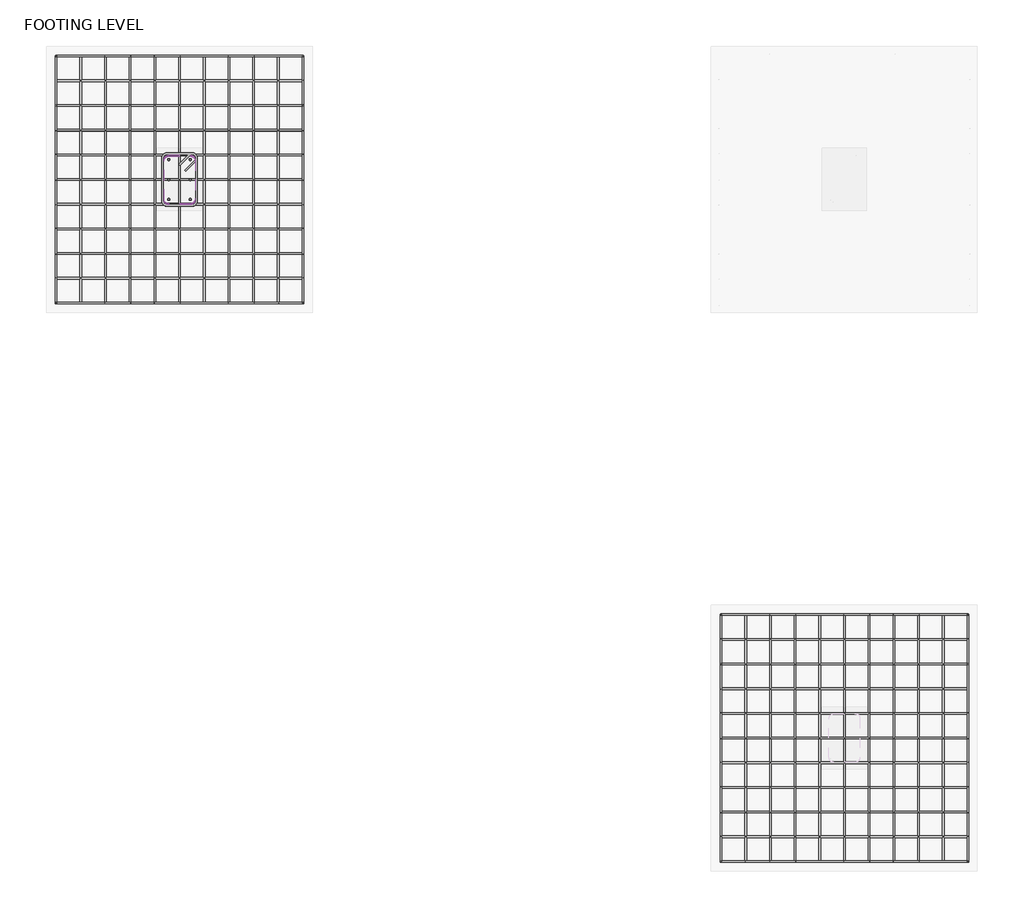
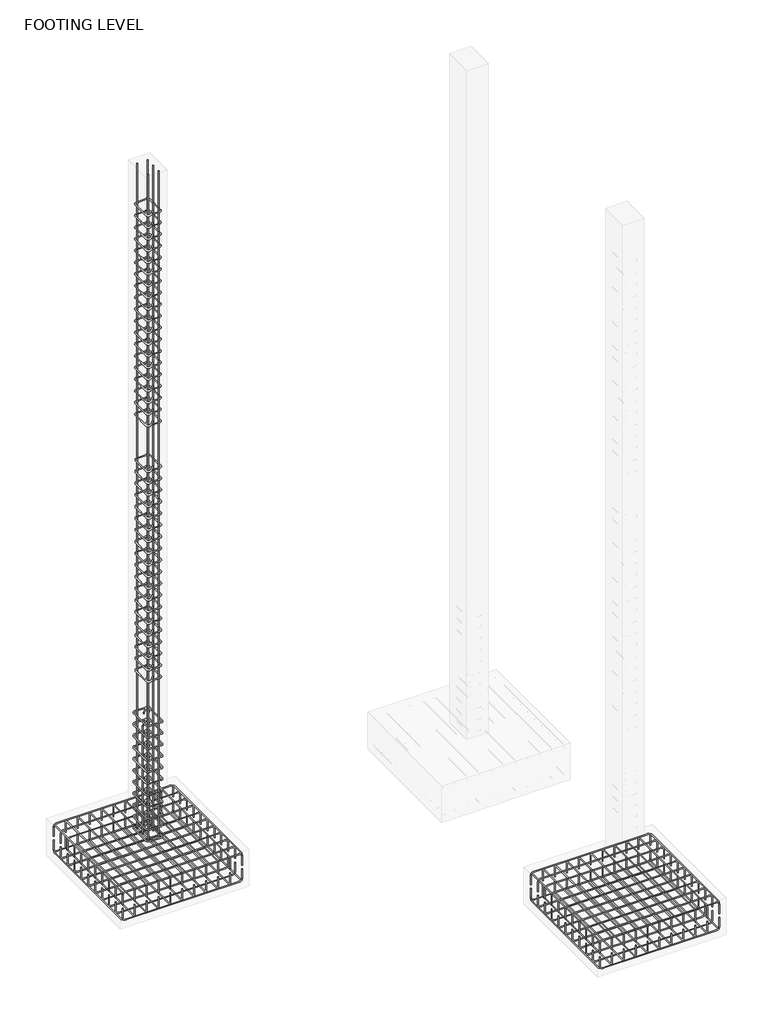
# One storey, part 2 of 9: 17 reinforcing bars.
"""IFC4 building model written with IfcOpenShell, lengths in millimetres."""

from ifc_helpers import new_model, si_unit, point, frame, origin, place, context, project, spatial, polyline, circle_curve, trimmed, segment, composite_curve, source, transform, mapped, element, save
from ifc_brep_helpers import swept_disk

model = new_model("IFC4")

# Units and contexts
model_context = context("Model", 3, world=origin())
ifc_project = project(units=[si_unit("LENGTHUNIT", "METRE", prefix="MILLI")], contexts=[model_context])

# Site, building, storey
site = spatial("IfcSite", under=ifc_project)
building = spatial("IfcBuilding", under=site)
storey = spatial("IfcBuildingStorey", under=building, Name="FOOTING LEVEL", Elevation=-1981.2)

# Reinforcing bars
placement = place(None, origin())
reinforcing_bar_shape = source(origin(), model_context, "Body", "SolidModel", [
    swept_disk(composite_curve([segment(polyline([(-7844.8521159, -3054.1904098, -2183.60625), (-7844.8521159, -3054.1904098, -2069.30625)]), True, "CONTINUOUS"), segment(trimmed(circle_curve(frame((-7844.8521159, -3087.5279098, -2069.30625), z_axis=(1.0, 0.0, 0.0), x_axis=(0.0, 33.33750000000009, 0.0)), 33.3375), [point((-7844.8521159, -3054.1904098, -2069.30625))], [point((-7844.8521159, -3087.5279098, -2035.96875))], True, "CARTESIAN"), True, "CONTINUOUS"), segment(polyline([(-7844.8521159, -3087.5279098, -2035.96875), (-7844.8521159, -4435.3154098, -2035.96875)]), True, "CONTINUOUS"), segment(trimmed(circle_curve(frame((-7844.8521159, -4435.3154098, -2069.30625), z_axis=(1.0, 0.0, 0.0), x_axis=(0.0, 0.0, 33.33750000000009)), 33.3375), [point((-7844.8521159, -4435.3154098, -2035.96875))], [point((-7844.8521159, -4468.6529098, -2069.30625))], True, "CARTESIAN"), True, "CONTINUOUS"), segment(polyline([(-7844.8521159, -4468.6529098, -2069.30625), (-7844.8521159, -4468.6529098, -2183.60625)]), True, "CONTINUOUS")], self_intersect=False), 4.7625),
])
element("IfcReinforcingBar", 1, at=placement, inside=storey, context=model_context, shape_type="MappedRepresentation", body=[
    mapped(reinforcing_bar_shape, transform((0.0, 0.0, 0.0), x_axis=(1.0, 0.0, 0.0), y_axis=(0.0, 1.0, 0.0), z_axis=(0.0, 0.0, 1.0))),
    mapped(reinforcing_bar_shape, transform((-141.44625, 0.0, 0.0), x_axis=(1.0, 0.0, 0.0), y_axis=(0.0, 1.0, 0.0), z_axis=(0.0, 0.0, 1.0))),
    mapped(reinforcing_bar_shape, transform((-282.8925, 0.0, 0.0), x_axis=(1.0, 0.0, 0.0), y_axis=(0.0, 1.0, 0.0), z_axis=(0.0, 0.0, 1.0))),
    mapped(reinforcing_bar_shape, transform((-424.33875, 0.0, 0.0), x_axis=(1.0, 0.0, 0.0), y_axis=(0.0, 1.0, 0.0), z_axis=(0.0, 0.0, 1.0))),
    mapped(reinforcing_bar_shape, transform((-565.785, 0.0, 0.0), x_axis=(1.0, 0.0, 0.0), y_axis=(0.0, 1.0, 0.0), z_axis=(0.0, 0.0, 1.0))),
    mapped(reinforcing_bar_shape, transform((-707.23125, 0.0, 0.0), x_axis=(1.0, 0.0, 0.0), y_axis=(0.0, 1.0, 0.0), z_axis=(0.0, 0.0, 1.0))),
    mapped(reinforcing_bar_shape, transform((-848.6775, 0.0, 0.0), x_axis=(1.0, 0.0, 0.0), y_axis=(0.0, 1.0, 0.0), z_axis=(0.0, 0.0, 1.0))),
    mapped(reinforcing_bar_shape, transform((-990.12375, 0.0, 0.0), x_axis=(1.0, 0.0, 0.0), y_axis=(0.0, 1.0, 0.0), z_axis=(0.0, 0.0, 1.0))),
    mapped(reinforcing_bar_shape, transform((-1131.57, 0.0, 0.0), x_axis=(1.0, 0.0, 0.0), y_axis=(0.0, 1.0, 0.0), z_axis=(0.0, 0.0, 1.0))),
    mapped(reinforcing_bar_shape, transform((-1273.01625, 0.0, 0.0), x_axis=(1.0, 0.0, 0.0), y_axis=(0.0, 1.0, 0.0), z_axis=(0.0, 0.0, 1.0))),
    mapped(reinforcing_bar_shape, transform((-1414.4625, 0.0, 0.0), x_axis=(1.0, 0.0, 0.0), y_axis=(0.0, 1.0, 0.0), z_axis=(0.0, 0.0, 1.0))),
])
reinforcing_bar_2_shape = source(origin(), model_context, "Body", "SolidModel", [
    swept_disk(composite_curve([segment(polyline([(-7844.8521159, -4468.6529098, -2235.99375), (-7844.8521159, -4468.6529098, -2350.29375)]), True, "CONTINUOUS"), segment(trimmed(circle_curve(frame((-7844.8521159, -4435.3154098, -2350.29375), z_axis=(1.0, 0.0, 0.0), x_axis=(0.0, -33.337499999999636, 0.0)), 33.3375), [point((-7844.8521159, -4468.6529098, -2350.29375))], [point((-7844.8521159, -4435.3154098, -2383.63125))], True, "CARTESIAN"), True, "CONTINUOUS"), segment(polyline([(-7844.8521159, -4435.3154098, -2383.63125), (-7844.8521159, -3087.5279098, -2383.63125)]), True, "CONTINUOUS"), segment(trimmed(circle_curve(frame((-7844.8521159, -3087.5279098, -2350.29375), z_axis=(1.0, 0.0, 0.0), x_axis=(0.0, 0.0, -33.33750000000009)), 33.3375), [point((-7844.8521159, -3087.5279098, -2383.63125))], [point((-7844.8521159, -3054.1904098, -2350.29375))], True, "CARTESIAN"), True, "CONTINUOUS"), segment(polyline([(-7844.8521159, -3054.1904098, -2350.29375), (-7844.8521159, -3054.1904098, -2235.99375)]), True, "CONTINUOUS")], self_intersect=False), 4.7625),
])
element("IfcReinforcingBar", 2, at=placement, inside=storey, context=model_context, shape_type="MappedRepresentation", body=[
    mapped(reinforcing_bar_2_shape, transform((0.0, 0.0, 0.0), x_axis=(1.0, 0.0, 0.0), y_axis=(0.0, 1.0, 0.0), z_axis=(0.0, 0.0, 1.0))),
    mapped(reinforcing_bar_2_shape, transform((-141.44625, 0.0, 0.0), x_axis=(1.0, 0.0, 0.0), y_axis=(0.0, 1.0, 0.0), z_axis=(0.0, 0.0, 1.0))),
    mapped(reinforcing_bar_2_shape, transform((-282.8925, 0.0, 0.0), x_axis=(1.0, 0.0, 0.0), y_axis=(0.0, 1.0, 0.0), z_axis=(0.0, 0.0, 1.0))),
    mapped(reinforcing_bar_2_shape, transform((-424.33875, 0.0, 0.0), x_axis=(1.0, 0.0, 0.0), y_axis=(0.0, 1.0, 0.0), z_axis=(0.0, 0.0, 1.0))),
    mapped(reinforcing_bar_2_shape, transform((-565.785, 0.0, 0.0), x_axis=(1.0, 0.0, 0.0), y_axis=(0.0, 1.0, 0.0), z_axis=(0.0, 0.0, 1.0))),
    mapped(reinforcing_bar_2_shape, transform((-707.23125, 0.0, 0.0), x_axis=(1.0, 0.0, 0.0), y_axis=(0.0, 1.0, 0.0), z_axis=(0.0, 0.0, 1.0))),
    mapped(reinforcing_bar_2_shape, transform((-848.6775, 0.0, 0.0), x_axis=(1.0, 0.0, 0.0), y_axis=(0.0, 1.0, 0.0), z_axis=(0.0, 0.0, 1.0))),
    mapped(reinforcing_bar_2_shape, transform((-990.12375, 0.0, 0.0), x_axis=(1.0, 0.0, 0.0), y_axis=(0.0, 1.0, 0.0), z_axis=(0.0, 0.0, 1.0))),
    mapped(reinforcing_bar_2_shape, transform((-1131.57, 0.0, 0.0), x_axis=(1.0, 0.0, 0.0), y_axis=(0.0, 1.0, 0.0), z_axis=(0.0, 0.0, 1.0))),
    mapped(reinforcing_bar_2_shape, transform((-1273.01625, 0.0, 0.0), x_axis=(1.0, 0.0, 0.0), y_axis=(0.0, 1.0, 0.0), z_axis=(0.0, 0.0, 1.0))),
    mapped(reinforcing_bar_2_shape, transform((-1414.4625, 0.0, 0.0), x_axis=(1.0, 0.0, 0.0), y_axis=(0.0, 1.0, 0.0), z_axis=(0.0, 0.0, 1.0))),
])
reinforcing_bar_3_shape = source(origin(), model_context, "Body", "SolidModel", [
    swept_disk(composite_curve([segment(polyline([(-9259.3146159, -3054.1904098, -2183.5650752), (-9259.3146159, -3054.1904098, -2069.2650752)]), True, "CONTINUOUS"), segment(trimmed(circle_curve(frame((-9225.9771159, -3054.1904098, -2069.2650752), z_axis=(0.0, 1.0, 0.0), x_axis=(-33.337500000001455, 0.0, 0.0)), 33.3375), [point((-9259.3146159, -3054.1904098, -2069.2650752))], [point((-9225.9771159, -3054.1904098, -2035.9275752))], True, "CARTESIAN"), True, "CONTINUOUS"), segment(polyline([(-9225.9771159, -3054.1904098, -2035.9275752), (-7878.1896159, -3054.1904098, -2035.9275752)]), True, "CONTINUOUS"), segment(trimmed(circle_curve(frame((-7878.1896159, -3054.1904098, -2069.2650752), z_axis=(0.0, 1.0, 0.0), x_axis=(0.0, 0.0, 33.337499999999864)), 33.3375), [point((-7878.1896159, -3054.1904098, -2035.9275752))], [point((-7844.8521159, -3054.1904098, -2069.2650752))], True, "CARTESIAN"), True, "CONTINUOUS"), segment(polyline([(-7844.8521159, -3054.1904098, -2069.2650752), (-7844.8521159, -3054.1904098, -2183.5650752)]), True, "CONTINUOUS")], self_intersect=False), 4.7625),
])
element("IfcReinforcingBar", 3, at=placement, inside=storey, context=model_context, shape_type="MappedRepresentation", body=[
    mapped(reinforcing_bar_3_shape, transform((0.0, 0.0, 0.0), x_axis=(1.0, 0.0, 0.0), y_axis=(0.0, 1.0, 0.0), z_axis=(0.0, 0.0, 1.0))),
    mapped(reinforcing_bar_3_shape, transform((0.0, -141.44625, 0.0), x_axis=(1.0, 0.0, 0.0), y_axis=(0.0, 1.0, 0.0), z_axis=(0.0, 0.0, 1.0))),
    mapped(reinforcing_bar_3_shape, transform((0.0, -282.8925, 0.0), x_axis=(1.0, 0.0, 0.0), y_axis=(0.0, 1.0, 0.0), z_axis=(0.0, 0.0, 1.0))),
    mapped(reinforcing_bar_3_shape, transform((0.0, -424.33875, 0.0), x_axis=(1.0, 0.0, 0.0), y_axis=(0.0, 1.0, 0.0), z_axis=(0.0, 0.0, 1.0))),
    mapped(reinforcing_bar_3_shape, transform((0.0, -565.785, 0.0), x_axis=(1.0, 0.0, 0.0), y_axis=(0.0, 1.0, 0.0), z_axis=(0.0, 0.0, 1.0))),
    mapped(reinforcing_bar_3_shape, transform((0.0, -707.23125, 0.0), x_axis=(1.0, 0.0, 0.0), y_axis=(0.0, 1.0, 0.0), z_axis=(0.0, 0.0, 1.0))),
    mapped(reinforcing_bar_3_shape, transform((0.0, -848.6775, 0.0), x_axis=(1.0, 0.0, 0.0), y_axis=(0.0, 1.0, 0.0), z_axis=(0.0, 0.0, 1.0))),
    mapped(reinforcing_bar_3_shape, transform((0.0, -990.12375, 0.0), x_axis=(1.0, 0.0, 0.0), y_axis=(0.0, 1.0, 0.0), z_axis=(0.0, 0.0, 1.0))),
    mapped(reinforcing_bar_3_shape, transform((0.0, -1131.57, 0.0), x_axis=(1.0, 0.0, 0.0), y_axis=(0.0, 1.0, 0.0), z_axis=(0.0, 0.0, 1.0))),
    mapped(reinforcing_bar_3_shape, transform((0.0, -1273.01625, 0.0), x_axis=(1.0, 0.0, 0.0), y_axis=(0.0, 1.0, 0.0), z_axis=(0.0, 0.0, 1.0))),
    mapped(reinforcing_bar_3_shape, transform((0.0, -1414.4625, 0.0), x_axis=(1.0, 0.0, 0.0), y_axis=(0.0, 1.0, 0.0), z_axis=(0.0, 0.0, 1.0))),
])
reinforcing_bar_4_shape = source(origin(), model_context, "Body", "SolidModel", [
    swept_disk(composite_curve([segment(polyline([(-9259.3146159, -4468.6529098, -2235.99375), (-9259.3146159, -4468.6529098, -2350.29375)]), True, "CONTINUOUS"), segment(trimmed(circle_curve(frame((-9225.9771159, -4468.6529098, -2350.29375), z_axis=(0.0, -1.0, 0.0), x_axis=(-33.337500000001455, 0.0, 0.0)), 33.3375), [point((-9259.3146159, -4468.6529098, -2350.29375))], [point((-9225.9771159, -4468.6529098, -2383.63125))], True, "CARTESIAN"), True, "CONTINUOUS"), segment(polyline([(-9225.9771159, -4468.6529098, -2383.63125), (-7878.1896159, -4468.6529098, -2383.63125)]), True, "CONTINUOUS"), segment(trimmed(circle_curve(frame((-7878.1896159, -4468.6529098, -2350.29375), z_axis=(0.0, -1.0, 0.0), x_axis=(0.0, 0.0, -33.33750000000009)), 33.3375), [point((-7878.1896159, -4468.6529098, -2383.63125))], [point((-7844.8521159, -4468.6529098, -2350.29375))], True, "CARTESIAN"), True, "CONTINUOUS"), segment(polyline([(-7844.8521159, -4468.6529098, -2350.29375), (-7844.8521159, -4468.6529098, -2235.99375)]), True, "CONTINUOUS")], self_intersect=False), 4.7625),
])
element("IfcReinforcingBar", 4, at=placement, inside=storey, context=model_context, shape_type="MappedRepresentation", body=[
    mapped(reinforcing_bar_4_shape, transform((0.0, 0.0, 0.0), x_axis=(1.0, 0.0, 0.0), y_axis=(0.0, 1.0, 0.0), z_axis=(0.0, 0.0, 1.0))),
    mapped(reinforcing_bar_4_shape, transform((0.0, 141.44625, 0.0), x_axis=(1.0, 0.0, 0.0), y_axis=(0.0, 1.0, 0.0), z_axis=(0.0, 0.0, 1.0))),
    mapped(reinforcing_bar_4_shape, transform((0.0, 282.8925, 0.0), x_axis=(1.0, 0.0, 0.0), y_axis=(0.0, 1.0, 0.0), z_axis=(0.0, 0.0, 1.0))),
    mapped(reinforcing_bar_4_shape, transform((0.0, 424.33875, 0.0), x_axis=(1.0, 0.0, 0.0), y_axis=(0.0, 1.0, 0.0), z_axis=(0.0, 0.0, 1.0))),
    mapped(reinforcing_bar_4_shape, transform((0.0, 565.785, 0.0), x_axis=(1.0, 0.0, 0.0), y_axis=(0.0, 1.0, 0.0), z_axis=(0.0, 0.0, 1.0))),
    mapped(reinforcing_bar_4_shape, transform((0.0, 707.23125, 0.0), x_axis=(1.0, 0.0, 0.0), y_axis=(0.0, 1.0, 0.0), z_axis=(0.0, 0.0, 1.0))),
    mapped(reinforcing_bar_4_shape, transform((0.0, 848.6775, 0.0), x_axis=(1.0, 0.0, 0.0), y_axis=(0.0, 1.0, 0.0), z_axis=(0.0, 0.0, 1.0))),
    mapped(reinforcing_bar_4_shape, transform((0.0, 990.12375, 0.0), x_axis=(1.0, 0.0, 0.0), y_axis=(0.0, 1.0, 0.0), z_axis=(0.0, 0.0, 1.0))),
    mapped(reinforcing_bar_4_shape, transform((0.0, 1131.57, 0.0), x_axis=(1.0, 0.0, 0.0), y_axis=(0.0, 1.0, 0.0), z_axis=(0.0, 0.0, 1.0))),
    mapped(reinforcing_bar_4_shape, transform((0.0, 1273.01625, 0.0), x_axis=(1.0, 0.0, 0.0), y_axis=(0.0, 1.0, 0.0), z_axis=(0.0, 0.0, 1.0))),
    mapped(reinforcing_bar_4_shape, transform((0.0, 1414.4625, 0.0), x_axis=(1.0, 0.0, 0.0), y_axis=(0.0, 1.0, 0.0), z_axis=(0.0, 0.0, 1.0))),
])
reinforcing_bar_5_shape = source(origin(), model_context, "Body", "SolidModel", [
    swept_disk(composite_curve([segment(polyline([(-11654.8521159, 146.2095902, -2183.60625), (-11654.8521159, 146.2095902, -2069.30625)]), True, "CONTINUOUS"), segment(trimmed(circle_curve(frame((-11654.8521159, 112.8720902, -2069.30625), z_axis=(1.0, 0.0, 0.0), x_axis=(0.0, 33.337500000000006, 0.0)), 33.3375), [point((-11654.8521159, 146.2095902, -2069.30625))], [point((-11654.8521159, 112.8720902, -2035.96875))], True, "CARTESIAN"), True, "CONTINUOUS"), segment(polyline([(-11654.8521159, 112.8720902, -2035.96875), (-11654.8521159, -1234.9154098, -2035.96875)]), True, "CONTINUOUS"), segment(trimmed(circle_curve(frame((-11654.8521159, -1234.9154098, -2069.30625), z_axis=(1.0, 0.0, 0.0), x_axis=(0.0, 0.0, 33.33750000000009)), 33.3375), [point((-11654.8521159, -1234.9154098, -2035.96875))], [point((-11654.8521159, -1268.2529098, -2069.30625))], True, "CARTESIAN"), True, "CONTINUOUS"), segment(polyline([(-11654.8521159, -1268.2529098, -2069.30625), (-11654.8521159, -1268.2529098, -2183.60625)]), True, "CONTINUOUS")], self_intersect=False), 4.7625),
])
element("IfcReinforcingBar", 5, at=placement, inside=storey, context=model_context, shape_type="MappedRepresentation", body=[
    mapped(reinforcing_bar_5_shape, transform((0.0, 0.0, 0.0), x_axis=(1.0, 0.0, 0.0), y_axis=(0.0, 1.0, 0.0), z_axis=(0.0, 0.0, 1.0))),
    mapped(reinforcing_bar_5_shape, transform((-141.44625, 0.0, 0.0), x_axis=(1.0, 0.0, 0.0), y_axis=(0.0, 1.0, 0.0), z_axis=(0.0, 0.0, 1.0))),
    mapped(reinforcing_bar_5_shape, transform((-282.8925, 0.0, 0.0), x_axis=(1.0, 0.0, 0.0), y_axis=(0.0, 1.0, 0.0), z_axis=(0.0, 0.0, 1.0))),
    mapped(reinforcing_bar_5_shape, transform((-424.33875, 0.0, 0.0), x_axis=(1.0, 0.0, 0.0), y_axis=(0.0, 1.0, 0.0), z_axis=(0.0, 0.0, 1.0))),
    mapped(reinforcing_bar_5_shape, transform((-565.785, 0.0, 0.0), x_axis=(1.0, 0.0, 0.0), y_axis=(0.0, 1.0, 0.0), z_axis=(0.0, 0.0, 1.0))),
    mapped(reinforcing_bar_5_shape, transform((-707.23125, 0.0, 0.0), x_axis=(1.0, 0.0, 0.0), y_axis=(0.0, 1.0, 0.0), z_axis=(0.0, 0.0, 1.0))),
    mapped(reinforcing_bar_5_shape, transform((-848.6775, 0.0, 0.0), x_axis=(1.0, 0.0, 0.0), y_axis=(0.0, 1.0, 0.0), z_axis=(0.0, 0.0, 1.0))),
    mapped(reinforcing_bar_5_shape, transform((-990.12375, 0.0, 0.0), x_axis=(1.0, 0.0, 0.0), y_axis=(0.0, 1.0, 0.0), z_axis=(0.0, 0.0, 1.0))),
    mapped(reinforcing_bar_5_shape, transform((-1131.57, 0.0, 0.0), x_axis=(1.0, 0.0, 0.0), y_axis=(0.0, 1.0, 0.0), z_axis=(0.0, 0.0, 1.0))),
    mapped(reinforcing_bar_5_shape, transform((-1273.01625, 0.0, 0.0), x_axis=(1.0, 0.0, 0.0), y_axis=(0.0, 1.0, 0.0), z_axis=(0.0, 0.0, 1.0))),
    mapped(reinforcing_bar_5_shape, transform((-1414.4625, 0.0, 0.0), x_axis=(1.0, 0.0, 0.0), y_axis=(0.0, 1.0, 0.0), z_axis=(0.0, 0.0, 1.0))),
])
reinforcing_bar_6_shape = source(origin(), model_context, "Body", "SolidModel", [
    swept_disk(composite_curve([segment(polyline([(-11654.8521159, -1268.2529098, -2235.99375), (-11654.8521159, -1268.2529098, -2350.29375)]), True, "CONTINUOUS"), segment(trimmed(circle_curve(frame((-11654.8521159, -1234.9154098, -2350.29375), z_axis=(1.0, 0.0, 0.0), x_axis=(0.0, -33.33750000000009, 0.0)), 33.3375), [point((-11654.8521159, -1268.2529098, -2350.29375))], [point((-11654.8521159, -1234.9154098, -2383.63125))], True, "CARTESIAN"), True, "CONTINUOUS"), segment(polyline([(-11654.8521159, -1234.9154098, -2383.63125), (-11654.8521159, 112.8720902, -2383.63125)]), True, "CONTINUOUS"), segment(trimmed(circle_curve(frame((-11654.8521159, 112.8720902, -2350.29375), z_axis=(1.0, 0.0, 0.0), x_axis=(0.0, 0.0, -33.33750000000009)), 33.3375), [point((-11654.8521159, 112.8720902, -2383.63125))], [point((-11654.8521159, 146.2095902, -2350.29375))], True, "CARTESIAN"), True, "CONTINUOUS"), segment(polyline([(-11654.8521159, 146.2095902, -2350.29375), (-11654.8521159, 146.2095902, -2235.99375)]), True, "CONTINUOUS")], self_intersect=False), 4.7625),
])
element("IfcReinforcingBar", 6, at=placement, inside=storey, context=model_context, shape_type="MappedRepresentation", body=[
    mapped(reinforcing_bar_6_shape, transform((0.0, 0.0, 0.0), x_axis=(1.0, 0.0, 0.0), y_axis=(0.0, 1.0, 0.0), z_axis=(0.0, 0.0, 1.0))),
    mapped(reinforcing_bar_6_shape, transform((-141.44625, 0.0, 0.0), x_axis=(1.0, 0.0, 0.0), y_axis=(0.0, 1.0, 0.0), z_axis=(0.0, 0.0, 1.0))),
    mapped(reinforcing_bar_6_shape, transform((-282.8925, 0.0, 0.0), x_axis=(1.0, 0.0, 0.0), y_axis=(0.0, 1.0, 0.0), z_axis=(0.0, 0.0, 1.0))),
    mapped(reinforcing_bar_6_shape, transform((-424.33875, 0.0, 0.0), x_axis=(1.0, 0.0, 0.0), y_axis=(0.0, 1.0, 0.0), z_axis=(0.0, 0.0, 1.0))),
    mapped(reinforcing_bar_6_shape, transform((-565.785, 0.0, 0.0), x_axis=(1.0, 0.0, 0.0), y_axis=(0.0, 1.0, 0.0), z_axis=(0.0, 0.0, 1.0))),
    mapped(reinforcing_bar_6_shape, transform((-707.23125, 0.0, 0.0), x_axis=(1.0, 0.0, 0.0), y_axis=(0.0, 1.0, 0.0), z_axis=(0.0, 0.0, 1.0))),
    mapped(reinforcing_bar_6_shape, transform((-848.6775, 0.0, 0.0), x_axis=(1.0, 0.0, 0.0), y_axis=(0.0, 1.0, 0.0), z_axis=(0.0, 0.0, 1.0))),
    mapped(reinforcing_bar_6_shape, transform((-990.12375, 0.0, 0.0), x_axis=(1.0, 0.0, 0.0), y_axis=(0.0, 1.0, 0.0), z_axis=(0.0, 0.0, 1.0))),
    mapped(reinforcing_bar_6_shape, transform((-1131.57, 0.0, 0.0), x_axis=(1.0, 0.0, 0.0), y_axis=(0.0, 1.0, 0.0), z_axis=(0.0, 0.0, 1.0))),
    mapped(reinforcing_bar_6_shape, transform((-1273.01625, 0.0, 0.0), x_axis=(1.0, 0.0, 0.0), y_axis=(0.0, 1.0, 0.0), z_axis=(0.0, 0.0, 1.0))),
    mapped(reinforcing_bar_6_shape, transform((-1414.4625, 0.0, 0.0), x_axis=(1.0, 0.0, 0.0), y_axis=(0.0, 1.0, 0.0), z_axis=(0.0, 0.0, 1.0))),
])
reinforcing_bar_7_shape = source(origin(), model_context, "Body", "SolidModel", [
    swept_disk(composite_curve([segment(polyline([(-13069.3146159, 146.2095902, -2183.5650752), (-13069.3146159, 146.2095902, -2069.2650752)]), True, "CONTINUOUS"), segment(trimmed(circle_curve(frame((-13035.9771159, 146.2095902, -2069.2650752), z_axis=(0.0, 1.0, 0.0), x_axis=(-33.337500000001455, 0.0, 0.0)), 33.3375), [point((-13069.3146159, 146.2095902, -2069.2650752))], [point((-13035.9771159, 146.2095902, -2035.9275752))], True, "CARTESIAN"), True, "CONTINUOUS"), segment(polyline([(-13035.9771159, 146.2095902, -2035.9275752), (-11688.1896159, 146.2095902, -2035.9275752)]), True, "CONTINUOUS"), segment(trimmed(circle_curve(frame((-11688.1896159, 146.2095902, -2069.2650752), z_axis=(0.0, 1.0, 0.0), x_axis=(0.0, 0.0, 33.337499999999864)), 33.3375), [point((-11688.1896159, 146.2095902, -2035.9275752))], [point((-11654.8521159, 146.2095902, -2069.2650752))], True, "CARTESIAN"), True, "CONTINUOUS"), segment(polyline([(-11654.8521159, 146.2095902, -2069.2650752), (-11654.8521159, 146.2095902, -2183.5650752)]), True, "CONTINUOUS")], self_intersect=False), 4.7625),
])
element("IfcReinforcingBar", 7, at=placement, inside=storey, context=model_context, shape_type="MappedRepresentation", body=[
    mapped(reinforcing_bar_7_shape, transform((0.0, 0.0, 0.0), x_axis=(1.0, 0.0, 0.0), y_axis=(0.0, 1.0, 0.0), z_axis=(0.0, 0.0, 1.0))),
    mapped(reinforcing_bar_7_shape, transform((0.0, -141.44625, 0.0), x_axis=(1.0, 0.0, 0.0), y_axis=(0.0, 1.0, 0.0), z_axis=(0.0, 0.0, 1.0))),
    mapped(reinforcing_bar_7_shape, transform((0.0, -282.8925, 0.0), x_axis=(1.0, 0.0, 0.0), y_axis=(0.0, 1.0, 0.0), z_axis=(0.0, 0.0, 1.0))),
    mapped(reinforcing_bar_7_shape, transform((0.0, -424.33875, 0.0), x_axis=(1.0, 0.0, 0.0), y_axis=(0.0, 1.0, 0.0), z_axis=(0.0, 0.0, 1.0))),
    mapped(reinforcing_bar_7_shape, transform((0.0, -565.785, 0.0), x_axis=(1.0, 0.0, 0.0), y_axis=(0.0, 1.0, 0.0), z_axis=(0.0, 0.0, 1.0))),
    mapped(reinforcing_bar_7_shape, transform((0.0, -707.23125, 0.0), x_axis=(1.0, 0.0, 0.0), y_axis=(0.0, 1.0, 0.0), z_axis=(0.0, 0.0, 1.0))),
    mapped(reinforcing_bar_7_shape, transform((0.0, -848.6775, 0.0), x_axis=(1.0, 0.0, 0.0), y_axis=(0.0, 1.0, 0.0), z_axis=(0.0, 0.0, 1.0))),
    mapped(reinforcing_bar_7_shape, transform((0.0, -990.12375, 0.0), x_axis=(1.0, 0.0, 0.0), y_axis=(0.0, 1.0, 0.0), z_axis=(0.0, 0.0, 1.0))),
    mapped(reinforcing_bar_7_shape, transform((0.0, -1131.57, 0.0), x_axis=(1.0, 0.0, 0.0), y_axis=(0.0, 1.0, 0.0), z_axis=(0.0, 0.0, 1.0))),
    mapped(reinforcing_bar_7_shape, transform((0.0, -1273.01625, 0.0), x_axis=(1.0, 0.0, 0.0), y_axis=(0.0, 1.0, 0.0), z_axis=(0.0, 0.0, 1.0))),
    mapped(reinforcing_bar_7_shape, transform((0.0, -1414.4625, 0.0), x_axis=(1.0, 0.0, 0.0), y_axis=(0.0, 1.0, 0.0), z_axis=(0.0, 0.0, 1.0))),
])
reinforcing_bar_8_shape = source(origin(), model_context, "Body", "SolidModel", [
    swept_disk(composite_curve([segment(polyline([(-13069.3146159, -1268.2529098, -2235.99375), (-13069.3146159, -1268.2529098, -2350.29375)]), True, "CONTINUOUS"), segment(trimmed(circle_curve(frame((-13035.9771159, -1268.2529098, -2350.29375), z_axis=(0.0, -1.0, 0.0), x_axis=(-33.337500000001455, 0.0, 0.0)), 33.3375), [point((-13069.3146159, -1268.2529098, -2350.29375))], [point((-13035.9771159, -1268.2529098, -2383.63125))], True, "CARTESIAN"), True, "CONTINUOUS"), segment(polyline([(-13035.9771159, -1268.2529098, -2383.63125), (-11688.1896159, -1268.2529098, -2383.63125)]), True, "CONTINUOUS"), segment(trimmed(circle_curve(frame((-11688.1896159, -1268.2529098, -2350.29375), z_axis=(0.0, -1.0, 0.0), x_axis=(0.0, 0.0, -33.33750000000009)), 33.3375), [point((-11688.1896159, -1268.2529098, -2383.63125))], [point((-11654.8521159, -1268.2529098, -2350.29375))], True, "CARTESIAN"), True, "CONTINUOUS"), segment(polyline([(-11654.8521159, -1268.2529098, -2350.29375), (-11654.8521159, -1268.2529098, -2235.99375)]), True, "CONTINUOUS")], self_intersect=False), 4.7625),
])
element("IfcReinforcingBar", 8, at=placement, inside=storey, context=model_context, shape_type="MappedRepresentation", body=[
    mapped(reinforcing_bar_8_shape, transform((0.0, 0.0, 0.0), x_axis=(1.0, 0.0, 0.0), y_axis=(0.0, 1.0, 0.0), z_axis=(0.0, 0.0, 1.0))),
    mapped(reinforcing_bar_8_shape, transform((0.0, 141.44625, 0.0), x_axis=(1.0, 0.0, 0.0), y_axis=(0.0, 1.0, 0.0), z_axis=(0.0, 0.0, 1.0))),
    mapped(reinforcing_bar_8_shape, transform((0.0, 282.8925, 0.0), x_axis=(1.0, 0.0, 0.0), y_axis=(0.0, 1.0, 0.0), z_axis=(0.0, 0.0, 1.0))),
    mapped(reinforcing_bar_8_shape, transform((0.0, 424.33875, 0.0), x_axis=(1.0, 0.0, 0.0), y_axis=(0.0, 1.0, 0.0), z_axis=(0.0, 0.0, 1.0))),
    mapped(reinforcing_bar_8_shape, transform((0.0, 565.785, 0.0), x_axis=(1.0, 0.0, 0.0), y_axis=(0.0, 1.0, 0.0), z_axis=(0.0, 0.0, 1.0))),
    mapped(reinforcing_bar_8_shape, transform((0.0, 707.23125, 0.0), x_axis=(1.0, 0.0, 0.0), y_axis=(0.0, 1.0, 0.0), z_axis=(0.0, 0.0, 1.0))),
    mapped(reinforcing_bar_8_shape, transform((0.0, 848.6775, 0.0), x_axis=(1.0, 0.0, 0.0), y_axis=(0.0, 1.0, 0.0), z_axis=(0.0, 0.0, 1.0))),
    mapped(reinforcing_bar_8_shape, transform((0.0, 990.12375, 0.0), x_axis=(1.0, 0.0, 0.0), y_axis=(0.0, 1.0, 0.0), z_axis=(0.0, 0.0, 1.0))),
    mapped(reinforcing_bar_8_shape, transform((0.0, 1131.57, 0.0), x_axis=(1.0, 0.0, 0.0), y_axis=(0.0, 1.0, 0.0), z_axis=(0.0, 0.0, 1.0))),
    mapped(reinforcing_bar_8_shape, transform((0.0, 1273.01625, 0.0), x_axis=(1.0, 0.0, 0.0), y_axis=(0.0, 1.0, 0.0), z_axis=(0.0, 0.0, 1.0))),
    mapped(reinforcing_bar_8_shape, transform((0.0, 1414.4625, 0.0), x_axis=(1.0, 0.0, 0.0), y_axis=(0.0, 1.0, 0.0), z_axis=(0.0, 0.0, 1.0))),
])
reinforcing_bar_9_shape = source(origin(), model_context, "Body", "SolidModel", [
    swept_disk(composite_curve([segment(polyline([(-12329.0845827, -510.8988371, -1951.0375), (-12272.2203857, -454.03464, -1951.0375)]), True, "CONTINUOUS"), segment(trimmed(circle_curve(frame((-12289.0583659, -437.1966598, -1951.0375), z_axis=(0.0, 0.0, 1.0), x_axis=(16.837980199999947, -16.837980200000004, 0.0)), 23.8125), [point((-12272.2203857, -454.03464, -1951.0375))], [point((-12289.0583659, -413.3841598, -1951.0375))], True, "CARTESIAN"), True, "CONTINUOUS"), segment(polyline([(-12289.0583659, -413.3841598, -1951.0375), (-12435.1083659, -413.3841598, -1951.0375)]), True, "CONTINUOUS"), segment(trimmed(circle_curve(frame((-12435.1083659, -437.1966598, -1951.0375), z_axis=(0.0, 0.0, 1.0), x_axis=(0.0, 23.8125, 0.0)), 23.8125), [point((-12435.1083659, -413.3841598, -1951.0375))], [point((-12458.9208659, -437.1966598, -1951.0375))], True, "CARTESIAN"), True, "CONTINUOUS"), segment(polyline([(-12458.9208659, -437.1966598, -1951.0375), (-12458.9208659, -684.8466598, -1951.0375)]), True, "CONTINUOUS"), segment(trimmed(circle_curve(frame((-12435.1371115, -684.8466598, -1952.2071928), z_axis=(0.04912095919979365, 0.0, 0.9987928370624672), x_axis=(-23.783754399999452, 0.0, 1.1696928000001208)), 23.8125), [point((-12458.9208659, -684.8466598, -1951.0375))], [point((-12435.1371115, -708.6591598, -1952.2071928))], True, "CARTESIAN"), True, "CONTINUOUS"), segment(polyline([(-12435.1371115, -708.6591598, -1952.2071928), (-12289.0296203, -708.6591598, -1959.3928072)]), True, "CONTINUOUS"), segment(trimmed(circle_curve(frame((-12289.0296203, -684.8466598, -1959.3928072), z_axis=(0.04912095919979365, 0.0, 0.9987928370624672), x_axis=(0.0, -23.8125, 0.0)), 23.8125), [point((-12289.0296203, -708.6591598, -1959.3928072))], [point((-12265.2458659, -684.8466598, -1960.5625))], True, "CARTESIAN"), True, "CONTINUOUS"), segment(polyline([(-12265.2458659, -684.8466598, -1960.5625), (-12265.2458659, -437.1966598, -1960.5625)]), True, "CONTINUOUS"), segment(trimmed(circle_curve(frame((-12289.0583659, -437.1966598, -1960.5625), z_axis=(0.0, 0.0, 1.0), x_axis=(23.8125, 0.0, 0.0)), 23.8125), [point((-12265.2458659, -437.1966598, -1960.5625))], [point((-12305.8963461, -420.3586796, -1960.5625))], True, "CARTESIAN"), True, "CONTINUOUS"), segment(polyline([(-12305.8963461, -420.3586796, -1960.5625), (-12362.7605432, -477.2228767, -1960.5625)]), True, "CONTINUOUS")], self_intersect=False), 4.7625),
])
element("IfcReinforcingBar", 9, at=placement, inside=storey, context=model_context, shape_type="MappedRepresentation", body=[
    mapped(reinforcing_bar_9_shape, transform((0.0, 0.0, 0.0), x_axis=(1.0, 0.0, 0.0), y_axis=(0.0, 1.0, 0.0), z_axis=(0.0, 0.0, 1.0))),
    mapped(reinforcing_bar_9_shape, transform((0.0, 0.0, 144.649777), x_axis=(1.0, 0.0, 0.0), y_axis=(0.0, 1.0, 0.0), z_axis=(0.0, 0.0, 1.0))),
    mapped(reinforcing_bar_9_shape, transform((0.0, 0.0, 289.299554), x_axis=(1.0, 0.0, 0.0), y_axis=(0.0, 1.0, 0.0), z_axis=(0.0, 0.0, 1.0))),
    mapped(reinforcing_bar_9_shape, transform((0.0, 0.0, 433.9493311), x_axis=(1.0, 0.0, 0.0), y_axis=(0.0, 1.0, 0.0), z_axis=(0.0, 0.0, 1.0))),
    mapped(reinforcing_bar_9_shape, transform((0.0, 0.0, 578.5991081), x_axis=(1.0, 0.0, 0.0), y_axis=(0.0, 1.0, 0.0), z_axis=(0.0, 0.0, 1.0))),
    mapped(reinforcing_bar_9_shape, transform((0.0, 0.0, 723.2488851), x_axis=(1.0, 0.0, 0.0), y_axis=(0.0, 1.0, 0.0), z_axis=(0.0, 0.0, 1.0))),
    mapped(reinforcing_bar_9_shape, transform((0.0, 0.0, 867.8986621), x_axis=(1.0, 0.0, 0.0), y_axis=(0.0, 1.0, 0.0), z_axis=(0.0, 0.0, 1.0))),
    mapped(reinforcing_bar_9_shape, transform((0.0, 0.0, 1012.5484392), x_axis=(1.0, 0.0, 0.0), y_axis=(0.0, 1.0, 0.0), z_axis=(0.0, 0.0, 1.0))),
    mapped(reinforcing_bar_9_shape, transform((0.0, 0.0, 1157.1982162), x_axis=(1.0, 0.0, 0.0), y_axis=(0.0, 1.0, 0.0), z_axis=(0.0, 0.0, 1.0))),
    mapped(reinforcing_bar_9_shape, transform((0.0, 0.0, 1301.8479932), x_axis=(1.0, 0.0, 0.0), y_axis=(0.0, 1.0, 0.0), z_axis=(0.0, 0.0, 1.0))),
    mapped(reinforcing_bar_9_shape, transform((0.0, 0.0, 1446.4977702), x_axis=(1.0, 0.0, 0.0), y_axis=(0.0, 1.0, 0.0), z_axis=(0.0, 0.0, 1.0))),
])
element("IfcReinforcingBar", 10, at=placement, inside=storey, context=model_context, shape_type="SolidModel", body=[
    swept_disk(composite_curve([segment(polyline([(-12300.2784581, -674.5029989, -1955.8), (-12300.2784581, -674.5029989, 6375.4)]), True, "CONTINUOUS")], self_intersect=False), 6.35),
])
element("IfcReinforcingBar", 11, at=placement, inside=storey, context=model_context, shape_type="SolidModel", body=[
    swept_disk(composite_curve([segment(polyline([(-12423.8882737, -674.5029989, -1955.8), (-12423.8882737, -674.5029989, 6375.4)]), True, "CONTINUOUS")], self_intersect=False), 6.35),
])
element("IfcReinforcingBar", 12, at=placement, inside=storey, context=model_context, shape_type="SolidModel", body=[
    swept_disk(composite_curve([segment(polyline([(-12300.2784581, -447.5403207, -1955.8), (-12300.2784581, -447.5403207, 6375.4)]), True, "CONTINUOUS")], self_intersect=False), 6.35),
])
element("IfcReinforcingBar", 13, at=placement, inside=storey, context=model_context, shape_type="SolidModel", body=[
    swept_disk(composite_curve([segment(polyline([(-12423.8882737, -447.5403207, -1955.8), (-12423.8882737, -447.5403207, 6375.4)]), True, "CONTINUOUS")], self_intersect=False), 6.35),
])
element("IfcReinforcingBar", 14, at=placement, inside=storey, context=model_context, shape_type="SolidModel", body=[
    swept_disk(composite_curve([segment(polyline([(-12300.2784581, -561.8403207, -1955.8), (-12300.2784581, -561.8403207, 6375.4)]), True, "CONTINUOUS")], self_intersect=False), 6.35),
])
element("IfcReinforcingBar", 15, at=placement, inside=storey, context=model_context, shape_type="SolidModel", body=[
    swept_disk(composite_curve([segment(polyline([(-12423.8882737, -561.8403207, -1955.8), (-12423.8882737, -561.8403207, -601.4305291)]), True, "CONTINUOUS")], self_intersect=False), 6.35),
])
reinforcing_bar_10_shape = source(origin(), model_context, "Body", "SolidModel", [
    swept_disk(composite_curve([segment(polyline([(-12382.3821491, -604.7944825, 42.8625), (-12439.2463461, -661.6586796, 42.8625)]), True, "CONTINUOUS"), segment(trimmed(circle_curve(frame((-12422.4083659, -678.4966598, 42.8625), z_axis=(0.0, 0.0, 1.0), x_axis=(-16.837980199999947, 16.837980199999947, 0.0)), 23.8125), [point((-12439.2463461, -661.6586796, 42.8625))], [point((-12422.4083659, -702.3091598, 42.8625))], True, "CARTESIAN"), True, "CONTINUOUS"), segment(polyline([(-12422.4083659, -702.3091598, 42.8625), (-12301.7583659, -702.3091598, 42.8625)]), True, "CONTINUOUS"), segment(trimmed(circle_curve(frame((-12301.7583659, -678.4966598, 42.8625), z_axis=(0.0, 0.0, 1.0), x_axis=(0.0, -23.8125, 0.0)), 23.8125), [point((-12301.7583659, -702.3091598, 42.8625))], [point((-12277.9458659, -678.4966598, 42.8625))], True, "CARTESIAN"), True, "CONTINUOUS"), segment(polyline([(-12277.9458659, -678.4966598, 42.8625), (-12277.9458659, -456.2466598, 42.8625)]), True, "CONTINUOUS"), segment(trimmed(circle_curve(frame((-12301.7203098, -456.2466598, 41.5167768), z_axis=(-0.056513312022656255, 0.0, 0.9984018457335854), x_axis=(23.774443900001643, 0.0, 1.3457231999999948)), 23.8125), [point((-12277.9458659, -456.2466598, 42.8625))], [point((-12301.7203098, -432.4341598, 41.5167768))], True, "CARTESIAN"), True, "CONTINUOUS"), segment(polyline([(-12301.7203098, -432.4341598, 41.5167768), (-12422.4464219, -432.4341598, 34.6832232)]), True, "CONTINUOUS"), segment(trimmed(circle_curve(frame((-12422.4464219, -456.2466598, 34.6832232), z_axis=(-0.056513312022656255, 0.0, 0.9984018457335854), x_axis=(0.0, 23.8125, 0.0)), 23.8125), [point((-12422.4464219, -432.4341598, 34.6832232))], [point((-12446.2208659, -456.2466598, 33.3375))], True, "CARTESIAN"), True, "CONTINUOUS"), segment(polyline([(-12446.2208659, -456.2466598, 33.3375), (-12446.2208659, -678.4966598, 33.3375)]), True, "CONTINUOUS"), segment(trimmed(circle_curve(frame((-12422.4083659, -678.4966598, 33.3375), z_axis=(0.0, 0.0, 1.0), x_axis=(-23.8125, 0.0, 0.0)), 23.8125), [point((-12446.2208659, -678.4966598, 33.3375))], [point((-12405.5703857, -695.33464, 33.3375))], True, "CARTESIAN"), True, "CONTINUOUS"), segment(polyline([(-12405.5703857, -695.33464, 33.3375), (-12348.7061886, -638.470443, 33.3375)]), True, "CONTINUOUS")], self_intersect=False), 4.7625),
])
element("IfcReinforcingBar", 16, at=placement, inside=storey, context=model_context, shape_type="MappedRepresentation", body=[
    mapped(reinforcing_bar_10_shape, transform((0.0, 0.0, 0.0), x_axis=(1.0, 0.0, 0.0), y_axis=(0.0, 1.0, 0.0), z_axis=(0.0, 0.0, 1.0))),
    mapped(reinforcing_bar_10_shape, transform((0.0, 0.0, 146.3515264), x_axis=(1.0, 0.0, 0.0), y_axis=(0.0, 1.0, 0.0), z_axis=(0.0, 0.0, 1.0))),
    mapped(reinforcing_bar_10_shape, transform((0.0, 0.0, 292.7030529), x_axis=(1.0, 0.0, 0.0), y_axis=(0.0, 1.0, 0.0), z_axis=(0.0, 0.0, 1.0))),
    mapped(reinforcing_bar_10_shape, transform((0.0, 0.0, 439.0545793), x_axis=(1.0, 0.0, 0.0), y_axis=(0.0, 1.0, 0.0), z_axis=(0.0, 0.0, 1.0))),
    mapped(reinforcing_bar_10_shape, transform((0.0, 0.0, 585.4061058), x_axis=(1.0, 0.0, 0.0), y_axis=(0.0, 1.0, 0.0), z_axis=(0.0, 0.0, 1.0))),
    mapped(reinforcing_bar_10_shape, transform((0.0, 0.0, 731.7576322), x_axis=(1.0, 0.0, 0.0), y_axis=(0.0, 1.0, 0.0), z_axis=(0.0, 0.0, 1.0))),
    mapped(reinforcing_bar_10_shape, transform((0.0, 0.0, 878.1091586), x_axis=(1.0, 0.0, 0.0), y_axis=(0.0, 1.0, 0.0), z_axis=(0.0, 0.0, 1.0))),
    mapped(reinforcing_bar_10_shape, transform((0.0, 0.0, 1024.4606851), x_axis=(1.0, 0.0, 0.0), y_axis=(0.0, 1.0, 0.0), z_axis=(0.0, 0.0, 1.0))),
    mapped(reinforcing_bar_10_shape, transform((0.0, 0.0, 1170.8122115), x_axis=(1.0, 0.0, 0.0), y_axis=(0.0, 1.0, 0.0), z_axis=(0.0, 0.0, 1.0))),
    mapped(reinforcing_bar_10_shape, transform((0.0, 0.0, 1317.163738), x_axis=(1.0, 0.0, 0.0), y_axis=(0.0, 1.0, 0.0), z_axis=(0.0, 0.0, 1.0))),
    mapped(reinforcing_bar_10_shape, transform((0.0, 0.0, 1463.5152644), x_axis=(1.0, 0.0, 0.0), y_axis=(0.0, 1.0, 0.0), z_axis=(0.0, 0.0, 1.0))),
    mapped(reinforcing_bar_10_shape, transform((0.0, 0.0, 1609.8667908), x_axis=(1.0, 0.0, 0.0), y_axis=(0.0, 1.0, 0.0), z_axis=(0.0, 0.0, 1.0))),
    mapped(reinforcing_bar_10_shape, transform((0.0, 0.0, 1756.2183173), x_axis=(1.0, 0.0, 0.0), y_axis=(0.0, 1.0, 0.0), z_axis=(0.0, 0.0, 1.0))),
    mapped(reinforcing_bar_10_shape, transform((0.0, 0.0, 1902.5698437), x_axis=(1.0, 0.0, 0.0), y_axis=(0.0, 1.0, 0.0), z_axis=(0.0, 0.0, 1.0))),
    mapped(reinforcing_bar_10_shape, transform((0.0, 0.0, 2048.9213702), x_axis=(1.0, 0.0, 0.0), y_axis=(0.0, 1.0, 0.0), z_axis=(0.0, 0.0, 1.0))),
    mapped(reinforcing_bar_10_shape, transform((0.0, 0.0, 2195.2728966), x_axis=(1.0, 0.0, 0.0), y_axis=(0.0, 1.0, 0.0), z_axis=(0.0, 0.0, 1.0))),
    mapped(reinforcing_bar_10_shape, transform((0.0, 0.0, 2341.6244231), x_axis=(1.0, 0.0, 0.0), y_axis=(0.0, 1.0, 0.0), z_axis=(0.0, 0.0, 1.0))),
    mapped(reinforcing_bar_10_shape, transform((0.0, 0.0, 2487.9759495), x_axis=(1.0, 0.0, 0.0), y_axis=(0.0, 1.0, 0.0), z_axis=(0.0, 0.0, 1.0))),
    mapped(reinforcing_bar_10_shape, transform((0.0, 0.0, 2634.3274759), x_axis=(1.0, 0.0, 0.0), y_axis=(0.0, 1.0, 0.0), z_axis=(0.0, 0.0, 1.0))),
])
reinforcing_bar_11_shape = source(origin(), model_context, "Body", "SolidModel", [
    swept_disk(composite_curve([segment(polyline([(-12382.3821491, -598.4444825, 3243.2625), (-12439.2463461, -655.3086796, 3243.2625)]), True, "CONTINUOUS"), segment(trimmed(circle_curve(frame((-12422.4083659, -672.1466598, 3243.2625), z_axis=(0.0, 0.0, 1.0), x_axis=(-16.837980199999947, 16.837980199999947, 0.0)), 23.8125), [point((-12439.2463461, -655.3086796, 3243.2625))], [point((-12422.4083659, -695.9591598, 3243.2625))], True, "CARTESIAN"), True, "CONTINUOUS"), segment(polyline([(-12422.4083659, -695.9591598, 3243.2625), (-12301.7583659, -695.9591598, 3243.2625)]), True, "CONTINUOUS"), segment(trimmed(circle_curve(frame((-12301.7583659, -672.1466598, 3243.2625), z_axis=(0.0, 0.0, 1.0), x_axis=(0.0, -23.8125, 0.0)), 23.8125), [point((-12301.7583659, -695.9591598, 3243.2625))], [point((-12277.9458659, -672.1466598, 3243.2625))], True, "CARTESIAN"), True, "CONTINUOUS"), segment(polyline([(-12277.9458659, -672.1466598, 3243.2625), (-12277.9458659, -449.8966598, 3243.2625)]), True, "CONTINUOUS"), segment(trimmed(circle_curve(frame((-12301.7203098, -449.8966598, 3241.9167768), z_axis=(-0.056513312022656255, 0.0, 0.9984018457335854), x_axis=(23.774443900001643, 0.0, 1.345723199999611)), 23.8125), [point((-12277.9458659, -449.8966598, 3243.2625))], [point((-12301.7203098, -426.0841598, 3241.9167768))], True, "CARTESIAN"), True, "CONTINUOUS"), segment(polyline([(-12301.7203098, -426.0841598, 3241.9167768), (-12422.4464219, -426.0841598, 3235.0832232)]), True, "CONTINUOUS"), segment(trimmed(circle_curve(frame((-12422.4464219, -449.8966598, 3235.0832232), z_axis=(-0.056513312022656255, 0.0, 0.9984018457335854), x_axis=(0.0, 23.8125, 0.0)), 23.8125), [point((-12422.4464219, -426.0841598, 3235.0832232))], [point((-12446.2208659, -449.8966598, 3233.7375))], True, "CARTESIAN"), True, "CONTINUOUS"), segment(polyline([(-12446.2208659, -449.8966598, 3233.7375), (-12446.2208659, -672.1466598, 3233.7375)]), True, "CONTINUOUS"), segment(trimmed(circle_curve(frame((-12422.4083659, -672.1466598, 3233.7375), z_axis=(0.0, 0.0, 1.0), x_axis=(-23.8125, 0.0, 0.0)), 23.8125), [point((-12446.2208659, -672.1466598, 3233.7375))], [point((-12405.5703857, -688.98464, 3233.7375))], True, "CARTESIAN"), True, "CONTINUOUS"), segment(polyline([(-12405.5703857, -688.98464, 3233.7375), (-12348.7061886, -632.120443, 3233.7375)]), True, "CONTINUOUS")], self_intersect=False), 4.7625),
])
element("IfcReinforcingBar", 17, at=placement, inside=storey, context=model_context, shape_type="MappedRepresentation", body=[
    mapped(reinforcing_bar_11_shape, transform((0.0, 0.0, 0.0), x_axis=(1.0, 0.0, 0.0), y_axis=(0.0, 1.0, 0.0), z_axis=(0.0, 0.0, 1.0))),
    mapped(reinforcing_bar_11_shape, transform((0.0, 0.0, 146.3443085), x_axis=(1.0, 0.0, 0.0), y_axis=(0.0, 1.0, 0.0), z_axis=(0.0, 0.0, 1.0))),
    mapped(reinforcing_bar_11_shape, transform((0.0, 0.0, 292.688617), x_axis=(1.0, 0.0, 0.0), y_axis=(0.0, 1.0, 0.0), z_axis=(0.0, 0.0, 1.0))),
    mapped(reinforcing_bar_11_shape, transform((0.0, 0.0, 439.0329255), x_axis=(1.0, 0.0, 0.0), y_axis=(0.0, 1.0, 0.0), z_axis=(0.0, 0.0, 1.0))),
    mapped(reinforcing_bar_11_shape, transform((0.0, 0.0, 585.377234), x_axis=(1.0, 0.0, 0.0), y_axis=(0.0, 1.0, 0.0), z_axis=(0.0, 0.0, 1.0))),
    mapped(reinforcing_bar_11_shape, transform((0.0, 0.0, 731.7215426), x_axis=(1.0, 0.0, 0.0), y_axis=(0.0, 1.0, 0.0), z_axis=(0.0, 0.0, 1.0))),
    mapped(reinforcing_bar_11_shape, transform((0.0, 0.0, 878.0658511), x_axis=(1.0, 0.0, 0.0), y_axis=(0.0, 1.0, 0.0), z_axis=(0.0, 0.0, 1.0))),
    mapped(reinforcing_bar_11_shape, transform((0.0, 0.0, 1024.4101596), x_axis=(1.0, 0.0, 0.0), y_axis=(0.0, 1.0, 0.0), z_axis=(0.0, 0.0, 1.0))),
    mapped(reinforcing_bar_11_shape, transform((0.0, 0.0, 1170.7544681), x_axis=(1.0, 0.0, 0.0), y_axis=(0.0, 1.0, 0.0), z_axis=(0.0, 0.0, 1.0))),
    mapped(reinforcing_bar_11_shape, transform((0.0, 0.0, 1317.0987766), x_axis=(1.0, 0.0, 0.0), y_axis=(0.0, 1.0, 0.0), z_axis=(0.0, 0.0, 1.0))),
    mapped(reinforcing_bar_11_shape, transform((0.0, 0.0, 1463.4430851), x_axis=(1.0, 0.0, 0.0), y_axis=(0.0, 1.0, 0.0), z_axis=(0.0, 0.0, 1.0))),
    mapped(reinforcing_bar_11_shape, transform((0.0, 0.0, 1609.7873936), x_axis=(1.0, 0.0, 0.0), y_axis=(0.0, 1.0, 0.0), z_axis=(0.0, 0.0, 1.0))),
    mapped(reinforcing_bar_11_shape, transform((0.0, 0.0, 1756.1317021), x_axis=(1.0, 0.0, 0.0), y_axis=(0.0, 1.0, 0.0), z_axis=(0.0, 0.0, 1.0))),
    mapped(reinforcing_bar_11_shape, transform((0.0, 0.0, 1902.4760106), x_axis=(1.0, 0.0, 0.0), y_axis=(0.0, 1.0, 0.0), z_axis=(0.0, 0.0, 1.0))),
    mapped(reinforcing_bar_11_shape, transform((0.0, 0.0, 2048.8203192), x_axis=(1.0, 0.0, 0.0), y_axis=(0.0, 1.0, 0.0), z_axis=(0.0, 0.0, 1.0))),
    mapped(reinforcing_bar_11_shape, transform((0.0, 0.0, 2195.1646277), x_axis=(1.0, 0.0, 0.0), y_axis=(0.0, 1.0, 0.0), z_axis=(0.0, 0.0, 1.0))),
    mapped(reinforcing_bar_11_shape, transform((0.0, 0.0, 2341.5089362), x_axis=(1.0, 0.0, 0.0), y_axis=(0.0, 1.0, 0.0), z_axis=(0.0, 0.0, 1.0))),
    mapped(reinforcing_bar_11_shape, transform((0.0, 0.0, 2487.8532447), x_axis=(1.0, 0.0, 0.0), y_axis=(0.0, 1.0, 0.0), z_axis=(0.0, 0.0, 1.0))),
    mapped(reinforcing_bar_11_shape, transform((0.0, 0.0, 2634.1975532), x_axis=(1.0, 0.0, 0.0), y_axis=(0.0, 1.0, 0.0), z_axis=(0.0, 0.0, 1.0))),
])

save(model, "model.ifc")

# Revit data of these elements
# Elements 1, 2, 3, 4, 5, 6, 7, 8, 9, 10, 11, 12, 13, 14, 15, 16, 17 (IfcReinforcingBar)
#   Phase Created = New Construction
